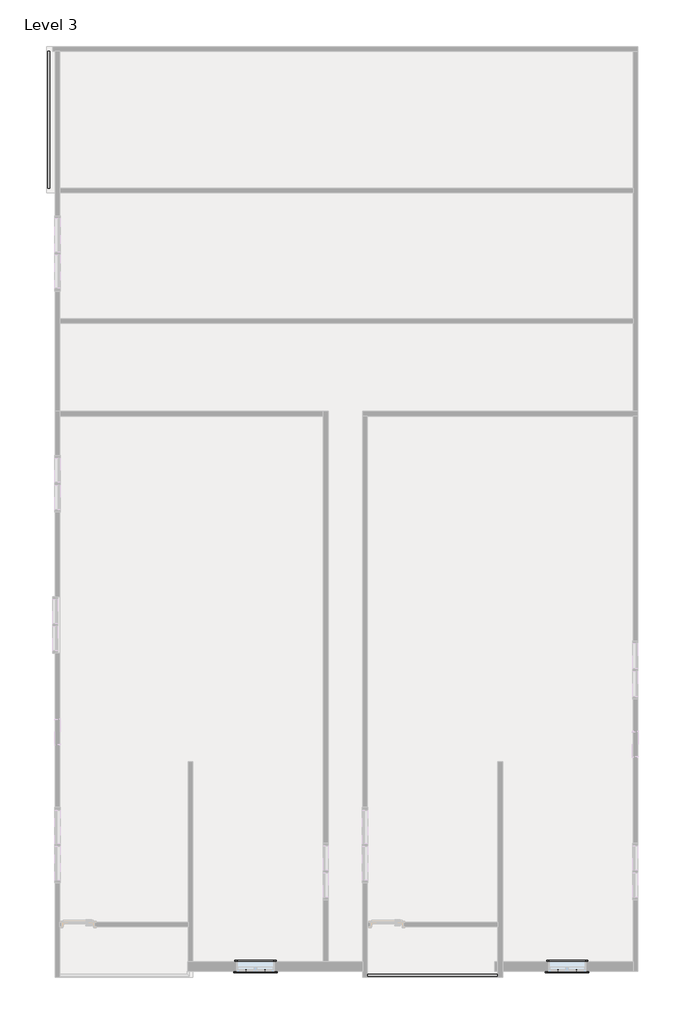
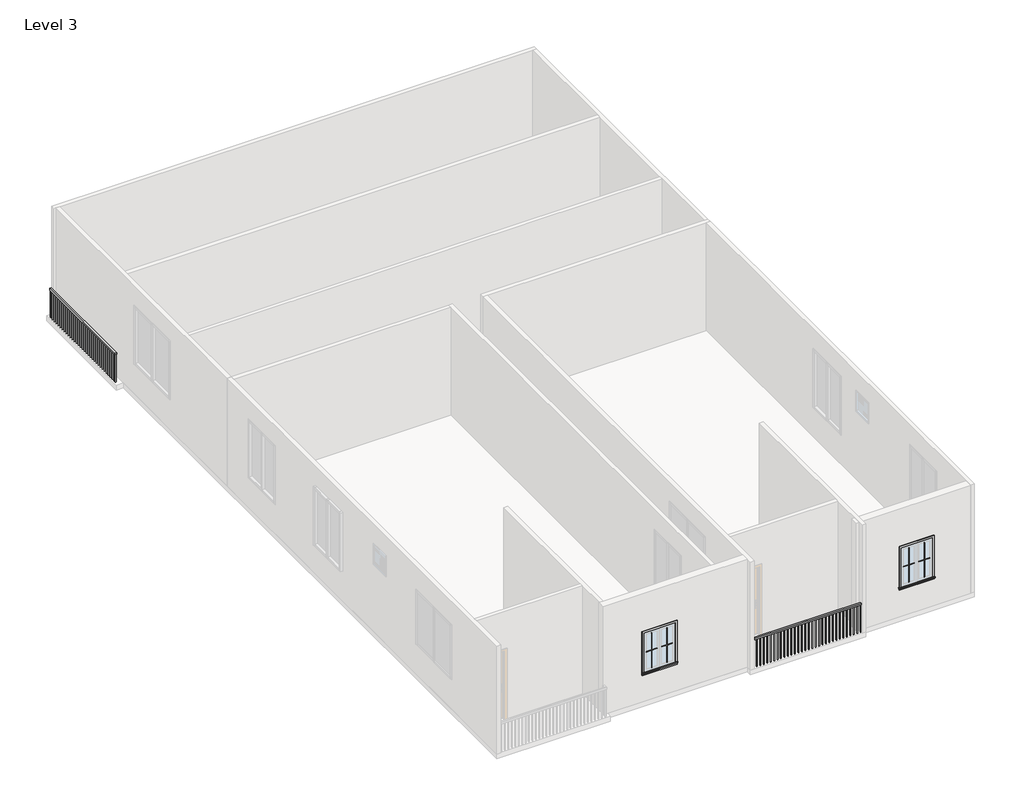
# One storey, part 3 of 3: 8 proxies, 3 railings.
"""IFC4 building model written with IfcOpenShell, lengths in millimetres."""

from ifc_helpers import new_model, si_unit, frame, origin, place, context, project, spatial, polyline, outline, extrude, transform, mapped, element, save
from components import muntin_pattern_2x2_muntin_pattern_2x2_1acec82f, muntin_pattern_2x2_muntin_pattern_2x2_43d02eee, trim_window_exterior_flat_with_sill_e4b28ec3, trim_window_interior_flat_picture_frame_39ff4276

model = new_model("IFC4")

# Units and contexts
model_context = context("Model", 3, world=origin())
ifc_project = project(units=[si_unit("LENGTHUNIT", "METRE", prefix="MILLI")], contexts=[model_context])

# Site, building, storey
site = spatial("IfcSite", under=ifc_project)
building = spatial("IfcBuilding", under=site)
storey = spatial("IfcBuildingStorey", under=building, Name="Level 3", Elevation=6705.6)

# Proxies
placement = place(None, origin())
muntin_pattern_2x2_muntin_pattern_2x2_shape = muntin_pattern_2x2_muntin_pattern_2x2_1acec82f(model_context)
element("IfcBuildingElementProxy", 1, Name="Muntin Pattern_2x2 : Muntin Pattern_2x2", ObjectType="Muntin Pattern_2x2 : Muntin Pattern_2x2", at=placement, inside=storey, context=model_context, shape_type="MappedRepresentation", body=[
    mapped(muntin_pattern_2x2_muntin_pattern_2x2_shape, transform((-3129.6612038, -10576.3529557, 7689.85), x_axis=(-1.0, 0.0, 0.0), y_axis=(0.0, -1.0, 0.0), z_axis=(0.0, 0.0, 1.0))),
])
element("IfcBuildingElementProxy", 2, Name="Muntin Pattern_2x2 : Muntin Pattern_2x2", ObjectType="Muntin Pattern_2x2 : Muntin Pattern_2x2", at=placement, inside=storey, context=model_context, shape_type="MappedRepresentation", body=[
    mapped(muntin_pattern_2x2_muntin_pattern_2x2_shape, transform((4424.1833786, -10576.3529557, 7689.85), x_axis=(-1.0, 0.0, 0.0), y_axis=(0.0, -1.0, 0.0), z_axis=(0.0, 0.0, 1.0))),
])
muntin_pattern_2x2_muntin_pattern_2x2_2_shape = muntin_pattern_2x2_muntin_pattern_2x2_43d02eee(model_context)
element("IfcBuildingElementProxy", 3, Name="Muntin Pattern_2x2 : Muntin Pattern_2x2", ObjectType="Muntin Pattern_2x2 : Muntin Pattern_2x2", at=placement, inside=storey, context=model_context, shape_type="MappedRepresentation", body=[
    mapped(muntin_pattern_2x2_muntin_pattern_2x2_2_shape, transform((-3583.6862038, -10576.3529557, 7689.85), x_axis=(1.0, 0.0, 0.0), y_axis=(0.0, 1.0, 0.0), z_axis=(0.0, 0.0, 1.0))),
])
element("IfcBuildingElementProxy", 4, Name="Muntin Pattern_2x2 : Muntin Pattern_2x2", ObjectType="Muntin Pattern_2x2 : Muntin Pattern_2x2", at=placement, inside=storey, context=model_context, shape_type="MappedRepresentation", body=[
    mapped(muntin_pattern_2x2_muntin_pattern_2x2_2_shape, transform((3970.1583786, -10576.3529557, 7689.85), x_axis=(1.0, 0.0, 0.0), y_axis=(0.0, 1.0, 0.0), z_axis=(0.0, 0.0, 1.0))),
])
trim_window_exterior_flat_with_sill_shape = trim_window_exterior_flat_with_sill_e4b28ec3(model_context)
element("IfcBuildingElementProxy", 5, Name="Trim-Window-Exterior-Flat : with Sill", ObjectType="Trim-Window-Exterior-Flat : with Sill", at=placement, inside=storey, context=model_context, shape_type="MappedRepresentation", body=[
    mapped(trim_window_exterior_flat_with_sill_shape, transform((-3356.6737038, -10585.8779557, 8839.2), x_axis=(1.0, 0.0, 0.0), y_axis=(0.0, 0.0, 1.0), z_axis=(0.0, -1.0, 0.0))),
])
element("IfcBuildingElementProxy", 6, Name="Trim-Window-Exterior-Flat : with Sill", ObjectType="Trim-Window-Exterior-Flat : with Sill", at=placement, inside=storey, context=model_context, shape_type="MappedRepresentation", body=[
    mapped(trim_window_exterior_flat_with_sill_shape, transform((4197.1708786, -10585.8779557, 8839.2), x_axis=(1.0, 0.0, 0.0), y_axis=(0.0, 0.0, 1.0), z_axis=(0.0, -1.0, 0.0))),
])
trim_window_interior_flat_picture_frame_shape = trim_window_interior_flat_picture_frame_39ff4276(model_context)
element("IfcBuildingElementProxy", 7, Name="Trim-Window-Interior-Flat : Picture Frame", ObjectType="Trim-Window-Interior-Flat : Picture Frame", at=placement, inside=storey, context=model_context, shape_type="MappedRepresentation", body=[
    mapped(trim_window_interior_flat_picture_frame_shape, transform((-3356.6737038, -10357.2779557, 8839.2), x_axis=(-1.0, 0.0, 0.0), y_axis=(0.0, 0.0, 1.0), z_axis=(0.0, 1.0, 0.0))),
])
element("IfcBuildingElementProxy", 8, Name="Trim-Window-Interior-Flat : Picture Frame", ObjectType="Trim-Window-Interior-Flat : Picture Frame", at=placement, inside=storey, context=model_context, shape_type="MappedRepresentation", body=[
    mapped(trim_window_interior_flat_picture_frame_shape, transform((4197.1708786, -10357.2779557, 8839.2), x_axis=(-1.0, 0.0, 0.0), y_axis=(0.0, 0.0, 1.0), z_axis=(0.0, 1.0, 0.0))),
])

# Railings
element("IfcRailing", 9, ObjectType="Handrail - Rectangular", at=placement, inside=storey, context=model_context, shape_type="SweptSolid", body=[
    extrude(outline(polyline([(-648.5431282, -10709.8005933), (-648.5431282, -10659.0005933), (2515.990751, -10659.0005933), (2515.990751, -10709.8005933), (-648.5431282, -10709.8005933)])), frame((0.0, 0.0, 7569.2), z_axis=(0.0, 0.0, 1.0), x_axis=(1.0, 0.0, 0.0)), (0.0, 0.0, 1.0), 50.8),
    extrude(outline(polyline([(2491.5318718, -10693.9255933), (2491.5318718, -10674.8755933), (2510.5818718, -10674.8755933), (2510.5818718, -10693.9255933), (2491.5318718, -10693.9255933)])), frame((0.0, 0.0, 6705.6), z_axis=(0.0, 0.0, 1.0), x_axis=(1.0, 0.0, 0.0)), (0.0, 0.0, 1.0), 863.6),
    extrude(outline(polyline([(2389.9318718, -10693.9255933), (2389.9318718, -10674.8755933), (2408.9818718, -10674.8755933), (2408.9818718, -10693.9255933), (2389.9318718, -10693.9255933)])), frame((0.0, 0.0, 6705.6), z_axis=(0.0, 0.0, 1.0), x_axis=(1.0, 0.0, 0.0)), (0.0, 0.0, 1.0), 863.6),
    extrude(outline(polyline([(2288.3318718, -10693.9255933), (2288.3318718, -10674.8755933), (2307.3818718, -10674.8755933), (2307.3818718, -10693.9255933), (2288.3318718, -10693.9255933)])), frame((0.0, 0.0, 6705.6), z_axis=(0.0, 0.0, 1.0), x_axis=(1.0, 0.0, 0.0)), (0.0, 0.0, 1.0), 863.6),
    extrude(outline(polyline([(2186.7318718, -10693.9255933), (2186.7318718, -10674.8755933), (2205.7818718, -10674.8755933), (2205.7818718, -10693.9255933), (2186.7318718, -10693.9255933)])), frame((0.0, 0.0, 6705.6), z_axis=(0.0, 0.0, 1.0), x_axis=(1.0, 0.0, 0.0)), (0.0, 0.0, 1.0), 863.6),
    extrude(outline(polyline([(2085.1318718, -10693.9255933), (2085.1318718, -10674.8755933), (2104.1818718, -10674.8755933), (2104.1818718, -10693.9255933), (2085.1318718, -10693.9255933)])), frame((0.0, 0.0, 6705.6), z_axis=(0.0, 0.0, 1.0), x_axis=(1.0, 0.0, 0.0)), (0.0, 0.0, 1.0), 863.6),
    extrude(outline(polyline([(1983.5318718, -10693.9255933), (1983.5318718, -10674.8755933), (2002.5818718, -10674.8755933), (2002.5818718, -10693.9255933), (1983.5318718, -10693.9255933)])), frame((0.0, 0.0, 6705.6), z_axis=(0.0, 0.0, 1.0), x_axis=(1.0, 0.0, 0.0)), (0.0, 0.0, 1.0), 863.6),
    extrude(outline(polyline([(1881.9318718, -10693.9255933), (1881.9318718, -10674.8755933), (1900.9818718, -10674.8755933), (1900.9818718, -10693.9255933), (1881.9318718, -10693.9255933)])), frame((0.0, 0.0, 6705.6), z_axis=(0.0, 0.0, 1.0), x_axis=(1.0, 0.0, 0.0)), (0.0, 0.0, 1.0), 863.6),
    extrude(outline(polyline([(1780.3318718, -10693.9255933), (1780.3318718, -10674.8755933), (1799.3818718, -10674.8755933), (1799.3818718, -10693.9255933), (1780.3318718, -10693.9255933)])), frame((0.0, 0.0, 6705.6), z_axis=(0.0, 0.0, 1.0), x_axis=(1.0, 0.0, 0.0)), (0.0, 0.0, 1.0), 863.6),
    extrude(outline(polyline([(1678.7318718, -10693.9255933), (1678.7318718, -10674.8755933), (1697.7818718, -10674.8755933), (1697.7818718, -10693.9255933), (1678.7318718, -10693.9255933)])), frame((0.0, 0.0, 6705.6), z_axis=(0.0, 0.0, 1.0), x_axis=(1.0, 0.0, 0.0)), (0.0, 0.0, 1.0), 863.6),
    extrude(outline(polyline([(1577.1318718, -10693.9255933), (1577.1318718, -10674.8755933), (1596.1818718, -10674.8755933), (1596.1818718, -10693.9255933), (1577.1318718, -10693.9255933)])), frame((0.0, 0.0, 6705.6), z_axis=(0.0, 0.0, 1.0), x_axis=(1.0, 0.0, 0.0)), (0.0, 0.0, 1.0), 863.6),
    extrude(outline(polyline([(1475.5318718, -10693.9255933), (1475.5318718, -10674.8755933), (1494.5818718, -10674.8755933), (1494.5818718, -10693.9255933), (1475.5318718, -10693.9255933)])), frame((0.0, 0.0, 6705.6), z_axis=(0.0, 0.0, 1.0), x_axis=(1.0, 0.0, 0.0)), (0.0, 0.0, 1.0), 863.6),
    extrude(outline(polyline([(1373.9318718, -10693.9255933), (1373.9318718, -10674.8755933), (1392.9818718, -10674.8755933), (1392.9818718, -10693.9255933), (1373.9318718, -10693.9255933)])), frame((0.0, 0.0, 6705.6), z_axis=(0.0, 0.0, 1.0), x_axis=(1.0, 0.0, 0.0)), (0.0, 0.0, 1.0), 863.6),
    extrude(outline(polyline([(1272.3318718, -10693.9255933), (1272.3318718, -10674.8755933), (1291.3818718, -10674.8755933), (1291.3818718, -10693.9255933), (1272.3318718, -10693.9255933)])), frame((0.0, 0.0, 6705.6), z_axis=(0.0, 0.0, 1.0), x_axis=(1.0, 0.0, 0.0)), (0.0, 0.0, 1.0), 863.6),
    extrude(outline(polyline([(1170.7318718, -10693.9255933), (1170.7318718, -10674.8755933), (1189.7818718, -10674.8755933), (1189.7818718, -10693.9255933), (1170.7318718, -10693.9255933)])), frame((0.0, 0.0, 6705.6), z_axis=(0.0, 0.0, 1.0), x_axis=(1.0, 0.0, 0.0)), (0.0, 0.0, 1.0), 863.6),
    extrude(outline(polyline([(1069.1318718, -10693.9255933), (1069.1318718, -10674.8755933), (1088.1818718, -10674.8755933), (1088.1818718, -10693.9255933), (1069.1318718, -10693.9255933)])), frame((0.0, 0.0, 6705.6), z_axis=(0.0, 0.0, 1.0), x_axis=(1.0, 0.0, 0.0)), (0.0, 0.0, 1.0), 863.6),
    extrude(outline(polyline([(967.5318718, -10693.9255933), (967.5318718, -10674.8755933), (986.5818718, -10674.8755933), (986.5818718, -10693.9255933), (967.5318718, -10693.9255933)])), frame((0.0, 0.0, 6705.6), z_axis=(0.0, 0.0, 1.0), x_axis=(1.0, 0.0, 0.0)), (0.0, 0.0, 1.0), 863.6),
    extrude(outline(polyline([(865.9318718, -10693.9255933), (865.9318718, -10674.8755933), (884.9818718, -10674.8755933), (884.9818718, -10693.9255933), (865.9318718, -10693.9255933)])), frame((0.0, 0.0, 6705.6), z_axis=(0.0, 0.0, 1.0), x_axis=(1.0, 0.0, 0.0)), (0.0, 0.0, 1.0), 863.6),
    extrude(outline(polyline([(764.3318718, -10693.9255933), (764.3318718, -10674.8755933), (783.3818718, -10674.8755933), (783.3818718, -10693.9255933), (764.3318718, -10693.9255933)])), frame((0.0, 0.0, 6705.6), z_axis=(0.0, 0.0, 1.0), x_axis=(1.0, 0.0, 0.0)), (0.0, 0.0, 1.0), 863.6),
    extrude(outline(polyline([(662.7318718, -10693.9255933), (662.7318718, -10674.8755933), (681.7818718, -10674.8755933), (681.7818718, -10693.9255933), (662.7318718, -10693.9255933)])), frame((0.0, 0.0, 6705.6), z_axis=(0.0, 0.0, 1.0), x_axis=(1.0, 0.0, 0.0)), (0.0, 0.0, 1.0), 863.6),
    extrude(outline(polyline([(561.1318718, -10693.9255933), (561.1318718, -10674.8755933), (580.1818718, -10674.8755933), (580.1818718, -10693.9255933), (561.1318718, -10693.9255933)])), frame((0.0, 0.0, 6705.6), z_axis=(0.0, 0.0, 1.0), x_axis=(1.0, 0.0, 0.0)), (0.0, 0.0, 1.0), 863.6),
    extrude(outline(polyline([(459.5318718, -10693.9255933), (459.5318718, -10674.8755933), (478.5818718, -10674.8755933), (478.5818718, -10693.9255933), (459.5318718, -10693.9255933)])), frame((0.0, 0.0, 6705.6), z_axis=(0.0, 0.0, 1.0), x_axis=(1.0, 0.0, 0.0)), (0.0, 0.0, 1.0), 863.6),
    extrude(outline(polyline([(357.9318718, -10693.9255933), (357.9318718, -10674.8755933), (376.9818718, -10674.8755933), (376.9818718, -10693.9255933), (357.9318718, -10693.9255933)])), frame((0.0, 0.0, 6705.6), z_axis=(0.0, 0.0, 1.0), x_axis=(1.0, 0.0, 0.0)), (0.0, 0.0, 1.0), 863.6),
    extrude(outline(polyline([(256.3318718, -10693.9255933), (256.3318718, -10674.8755933), (275.3818718, -10674.8755933), (275.3818718, -10693.9255933), (256.3318718, -10693.9255933)])), frame((0.0, 0.0, 6705.6), z_axis=(0.0, 0.0, 1.0), x_axis=(1.0, 0.0, 0.0)), (0.0, 0.0, 1.0), 863.6),
    extrude(outline(polyline([(154.7318718, -10693.9255933), (154.7318718, -10674.8755933), (173.7818718, -10674.8755933), (173.7818718, -10693.9255933), (154.7318718, -10693.9255933)])), frame((0.0, 0.0, 6705.6), z_axis=(0.0, 0.0, 1.0), x_axis=(1.0, 0.0, 0.0)), (0.0, 0.0, 1.0), 863.6),
    extrude(outline(polyline([(53.1318718, -10693.9255933), (53.1318718, -10674.8755933), (72.1818718, -10674.8755933), (72.1818718, -10693.9255933), (53.1318718, -10693.9255933)])), frame((0.0, 0.0, 6705.6), z_axis=(0.0, 0.0, 1.0), x_axis=(1.0, 0.0, 0.0)), (0.0, 0.0, 1.0), 863.6),
    extrude(outline(polyline([(-48.4681282, -10693.9255933), (-48.4681282, -10674.8755933), (-29.4181282, -10674.8755933), (-29.4181282, -10693.9255933), (-48.4681282, -10693.9255933)])), frame((0.0, 0.0, 6705.6), z_axis=(0.0, 0.0, 1.0), x_axis=(1.0, 0.0, 0.0)), (0.0, 0.0, 1.0), 863.6),
    extrude(outline(polyline([(-150.0681282, -10693.9255933), (-150.0681282, -10674.8755933), (-131.0181282, -10674.8755933), (-131.0181282, -10693.9255933), (-150.0681282, -10693.9255933)])), frame((0.0, 0.0, 6705.6), z_axis=(0.0, 0.0, 1.0), x_axis=(1.0, 0.0, 0.0)), (0.0, 0.0, 1.0), 863.6),
    extrude(outline(polyline([(-251.6681282, -10693.9255933), (-251.6681282, -10674.8755933), (-232.6181282, -10674.8755933), (-232.6181282, -10693.9255933), (-251.6681282, -10693.9255933)])), frame((0.0, 0.0, 6705.6), z_axis=(0.0, 0.0, 1.0), x_axis=(1.0, 0.0, 0.0)), (0.0, 0.0, 1.0), 863.6),
    extrude(outline(polyline([(-353.2681282, -10693.9255933), (-353.2681282, -10674.8755933), (-334.2181282, -10674.8755933), (-334.2181282, -10693.9255933), (-353.2681282, -10693.9255933)])), frame((0.0, 0.0, 6705.6), z_axis=(0.0, 0.0, 1.0), x_axis=(1.0, 0.0, 0.0)), (0.0, 0.0, 1.0), 863.6),
    extrude(outline(polyline([(-454.8681282, -10693.9255933), (-454.8681282, -10674.8755933), (-435.8181282, -10674.8755933), (-435.8181282, -10693.9255933), (-454.8681282, -10693.9255933)])), frame((0.0, 0.0, 6705.6), z_axis=(0.0, 0.0, 1.0), x_axis=(1.0, 0.0, 0.0)), (0.0, 0.0, 1.0), 863.6),
    extrude(outline(polyline([(-556.4681282, -10693.9255933), (-556.4681282, -10674.8755933), (-537.4181282, -10674.8755933), (-537.4181282, -10693.9255933), (-556.4681282, -10693.9255933)])), frame((0.0, 0.0, 6705.6), z_axis=(0.0, 0.0, 1.0), x_axis=(1.0, 0.0, 0.0)), (0.0, 0.0, 1.0), 863.6),
    extrude(outline(polyline([(2496.940751, -10693.9255933), (2496.940751, -10674.8755933), (2515.990751, -10674.8755933), (2515.990751, -10693.9255933), (2496.940751, -10693.9255933)])), frame((0.0, 0.0, 6705.6), z_axis=(0.0, 0.0, 1.0), x_axis=(1.0, 0.0, 0.0)), (0.0, 0.0, 1.0), 863.6),
    extrude(outline(polyline([(-648.5431282, -10693.9255933), (-648.5431282, -10674.8755933), (-629.4931282, -10674.8755933), (-629.4931282, -10693.9255933), (-648.5431282, -10693.9255933)])), frame((0.0, 0.0, 6705.6), z_axis=(0.0, 0.0, 1.0), x_axis=(1.0, 0.0, 0.0)), (0.0, 0.0, 1.0), 863.6),
])
element("IfcRailing", 10, ObjectType="Handrail - Rectangular", at=placement, inside=storey, context=model_context, shape_type="SweptSolid", body=[
    extrude(outline(polyline([(-8391.7551246, 11703.9189683), (-8340.9551246, 11703.9189683), (-8340.9551246, 8387.4224771), (-8391.7551246, 8387.4224771), (-8391.7551246, 11703.9189683)])), frame((0.0, 0.0, 7569.2), z_axis=(0.0, 0.0, 1.0), x_axis=(1.0, 0.0, 0.0)), (0.0, 0.0, 1.0), 50.8),
    extrude(outline(polyline([(-8375.8801246, 8462.2439683), (-8356.8301246, 8462.2439683), (-8356.8301246, 8443.1939683), (-8375.8801246, 8443.1939683), (-8375.8801246, 8462.2439683)])), frame((0.0, 0.0, 6705.6), z_axis=(0.0, 0.0, 1.0), x_axis=(1.0, 0.0, 0.0)), (0.0, 0.0, 1.0), 863.6),
    extrude(outline(polyline([(-8375.8801246, 8563.8439683), (-8356.8301246, 8563.8439683), (-8356.8301246, 8544.7939683), (-8375.8801246, 8544.7939683), (-8375.8801246, 8563.8439683)])), frame((0.0, 0.0, 6705.6), z_axis=(0.0, 0.0, 1.0), x_axis=(1.0, 0.0, 0.0)), (0.0, 0.0, 1.0), 863.6),
    extrude(outline(polyline([(-8375.8801246, 8665.4439683), (-8356.8301246, 8665.4439683), (-8356.8301246, 8646.3939683), (-8375.8801246, 8646.3939683), (-8375.8801246, 8665.4439683)])), frame((0.0, 0.0, 6705.6), z_axis=(0.0, 0.0, 1.0), x_axis=(1.0, 0.0, 0.0)), (0.0, 0.0, 1.0), 863.6),
    extrude(outline(polyline([(-8375.8801246, 8767.0439683), (-8356.8301246, 8767.0439683), (-8356.8301246, 8747.9939683), (-8375.8801246, 8747.9939683), (-8375.8801246, 8767.0439683)])), frame((0.0, 0.0, 6705.6), z_axis=(0.0, 0.0, 1.0), x_axis=(1.0, 0.0, 0.0)), (0.0, 0.0, 1.0), 863.6),
    extrude(outline(polyline([(-8375.8801246, 8868.6439683), (-8356.8301246, 8868.6439683), (-8356.8301246, 8849.5939683), (-8375.8801246, 8849.5939683), (-8375.8801246, 8868.6439683)])), frame((0.0, 0.0, 6705.6), z_axis=(0.0, 0.0, 1.0), x_axis=(1.0, 0.0, 0.0)), (0.0, 0.0, 1.0), 863.6),
    extrude(outline(polyline([(-8375.8801246, 8970.2439683), (-8356.8301246, 8970.2439683), (-8356.8301246, 8951.1939683), (-8375.8801246, 8951.1939683), (-8375.8801246, 8970.2439683)])), frame((0.0, 0.0, 6705.6), z_axis=(0.0, 0.0, 1.0), x_axis=(1.0, 0.0, 0.0)), (0.0, 0.0, 1.0), 863.6),
    extrude(outline(polyline([(-8375.8801246, 9071.8439683), (-8356.8301246, 9071.8439683), (-8356.8301246, 9052.7939683), (-8375.8801246, 9052.7939683), (-8375.8801246, 9071.8439683)])), frame((0.0, 0.0, 6705.6), z_axis=(0.0, 0.0, 1.0), x_axis=(1.0, 0.0, 0.0)), (0.0, 0.0, 1.0), 863.6),
    extrude(outline(polyline([(-8375.8801246, 9173.4439683), (-8356.8301246, 9173.4439683), (-8356.8301246, 9154.3939683), (-8375.8801246, 9154.3939683), (-8375.8801246, 9173.4439683)])), frame((0.0, 0.0, 6705.6), z_axis=(0.0, 0.0, 1.0), x_axis=(1.0, 0.0, 0.0)), (0.0, 0.0, 1.0), 863.6),
    extrude(outline(polyline([(-8375.8801246, 9275.0439683), (-8356.8301246, 9275.0439683), (-8356.8301246, 9255.9939683), (-8375.8801246, 9255.9939683), (-8375.8801246, 9275.0439683)])), frame((0.0, 0.0, 6705.6), z_axis=(0.0, 0.0, 1.0), x_axis=(1.0, 0.0, 0.0)), (0.0, 0.0, 1.0), 863.6),
    extrude(outline(polyline([(-8375.8801246, 9376.6439683), (-8356.8301246, 9376.6439683), (-8356.8301246, 9357.5939683), (-8375.8801246, 9357.5939683), (-8375.8801246, 9376.6439683)])), frame((0.0, 0.0, 6705.6), z_axis=(0.0, 0.0, 1.0), x_axis=(1.0, 0.0, 0.0)), (0.0, 0.0, 1.0), 863.6),
    extrude(outline(polyline([(-8375.8801246, 9478.2439683), (-8356.8301246, 9478.2439683), (-8356.8301246, 9459.1939683), (-8375.8801246, 9459.1939683), (-8375.8801246, 9478.2439683)])), frame((0.0, 0.0, 6705.6), z_axis=(0.0, 0.0, 1.0), x_axis=(1.0, 0.0, 0.0)), (0.0, 0.0, 1.0), 863.6),
    extrude(outline(polyline([(-8375.8801246, 9579.8439683), (-8356.8301246, 9579.8439683), (-8356.8301246, 9560.7939683), (-8375.8801246, 9560.7939683), (-8375.8801246, 9579.8439683)])), frame((0.0, 0.0, 6705.6), z_axis=(0.0, 0.0, 1.0), x_axis=(1.0, 0.0, 0.0)), (0.0, 0.0, 1.0), 863.6),
    extrude(outline(polyline([(-8375.8801246, 9681.4439683), (-8356.8301246, 9681.4439683), (-8356.8301246, 9662.3939683), (-8375.8801246, 9662.3939683), (-8375.8801246, 9681.4439683)])), frame((0.0, 0.0, 6705.6), z_axis=(0.0, 0.0, 1.0), x_axis=(1.0, 0.0, 0.0)), (0.0, 0.0, 1.0), 863.6),
    extrude(outline(polyline([(-8375.8801246, 9783.0439683), (-8356.8301246, 9783.0439683), (-8356.8301246, 9763.9939683), (-8375.8801246, 9763.9939683), (-8375.8801246, 9783.0439683)])), frame((0.0, 0.0, 6705.6), z_axis=(0.0, 0.0, 1.0), x_axis=(1.0, 0.0, 0.0)), (0.0, 0.0, 1.0), 863.6),
    extrude(outline(polyline([(-8375.8801246, 9884.6439683), (-8356.8301246, 9884.6439683), (-8356.8301246, 9865.5939683), (-8375.8801246, 9865.5939683), (-8375.8801246, 9884.6439683)])), frame((0.0, 0.0, 6705.6), z_axis=(0.0, 0.0, 1.0), x_axis=(1.0, 0.0, 0.0)), (0.0, 0.0, 1.0), 863.6),
    extrude(outline(polyline([(-8375.8801246, 9986.2439683), (-8356.8301246, 9986.2439683), (-8356.8301246, 9967.1939683), (-8375.8801246, 9967.1939683), (-8375.8801246, 9986.2439683)])), frame((0.0, 0.0, 6705.6), z_axis=(0.0, 0.0, 1.0), x_axis=(1.0, 0.0, 0.0)), (0.0, 0.0, 1.0), 863.6),
    extrude(outline(polyline([(-8375.8801246, 10087.8439683), (-8356.8301246, 10087.8439683), (-8356.8301246, 10068.7939683), (-8375.8801246, 10068.7939683), (-8375.8801246, 10087.8439683)])), frame((0.0, 0.0, 6705.6), z_axis=(0.0, 0.0, 1.0), x_axis=(1.0, 0.0, 0.0)), (0.0, 0.0, 1.0), 863.6),
    extrude(outline(polyline([(-8375.8801246, 10189.4439683), (-8356.8301246, 10189.4439683), (-8356.8301246, 10170.3939683), (-8375.8801246, 10170.3939683), (-8375.8801246, 10189.4439683)])), frame((0.0, 0.0, 6705.6), z_axis=(0.0, 0.0, 1.0), x_axis=(1.0, 0.0, 0.0)), (0.0, 0.0, 1.0), 863.6),
    extrude(outline(polyline([(-8375.8801246, 10291.0439683), (-8356.8301246, 10291.0439683), (-8356.8301246, 10271.9939683), (-8375.8801246, 10271.9939683), (-8375.8801246, 10291.0439683)])), frame((0.0, 0.0, 6705.6), z_axis=(0.0, 0.0, 1.0), x_axis=(1.0, 0.0, 0.0)), (0.0, 0.0, 1.0), 863.6),
    extrude(outline(polyline([(-8375.8801246, 10392.6439683), (-8356.8301246, 10392.6439683), (-8356.8301246, 10373.5939683), (-8375.8801246, 10373.5939683), (-8375.8801246, 10392.6439683)])), frame((0.0, 0.0, 6705.6), z_axis=(0.0, 0.0, 1.0), x_axis=(1.0, 0.0, 0.0)), (0.0, 0.0, 1.0), 863.6),
    extrude(outline(polyline([(-8375.8801246, 10494.2439683), (-8356.8301246, 10494.2439683), (-8356.8301246, 10475.1939683), (-8375.8801246, 10475.1939683), (-8375.8801246, 10494.2439683)])), frame((0.0, 0.0, 6705.6), z_axis=(0.0, 0.0, 1.0), x_axis=(1.0, 0.0, 0.0)), (0.0, 0.0, 1.0), 863.6),
    extrude(outline(polyline([(-8375.8801246, 10595.8439683), (-8356.8301246, 10595.8439683), (-8356.8301246, 10576.7939683), (-8375.8801246, 10576.7939683), (-8375.8801246, 10595.8439683)])), frame((0.0, 0.0, 6705.6), z_axis=(0.0, 0.0, 1.0), x_axis=(1.0, 0.0, 0.0)), (0.0, 0.0, 1.0), 863.6),
    extrude(outline(polyline([(-8375.8801246, 10697.4439683), (-8356.8301246, 10697.4439683), (-8356.8301246, 10678.3939683), (-8375.8801246, 10678.3939683), (-8375.8801246, 10697.4439683)])), frame((0.0, 0.0, 6705.6), z_axis=(0.0, 0.0, 1.0), x_axis=(1.0, 0.0, 0.0)), (0.0, 0.0, 1.0), 863.6),
    extrude(outline(polyline([(-8375.8801246, 10799.0439683), (-8356.8301246, 10799.0439683), (-8356.8301246, 10779.9939683), (-8375.8801246, 10779.9939683), (-8375.8801246, 10799.0439683)])), frame((0.0, 0.0, 6705.6), z_axis=(0.0, 0.0, 1.0), x_axis=(1.0, 0.0, 0.0)), (0.0, 0.0, 1.0), 863.6),
    extrude(outline(polyline([(-8375.8801246, 10900.6439683), (-8356.8301246, 10900.6439683), (-8356.8301246, 10881.5939683), (-8375.8801246, 10881.5939683), (-8375.8801246, 10900.6439683)])), frame((0.0, 0.0, 6705.6), z_axis=(0.0, 0.0, 1.0), x_axis=(1.0, 0.0, 0.0)), (0.0, 0.0, 1.0), 863.6),
    extrude(outline(polyline([(-8375.8801246, 11002.2439683), (-8356.8301246, 11002.2439683), (-8356.8301246, 10983.1939683), (-8375.8801246, 10983.1939683), (-8375.8801246, 11002.2439683)])), frame((0.0, 0.0, 6705.6), z_axis=(0.0, 0.0, 1.0), x_axis=(1.0, 0.0, 0.0)), (0.0, 0.0, 1.0), 863.6),
    extrude(outline(polyline([(-8375.8801246, 11103.8439683), (-8356.8301246, 11103.8439683), (-8356.8301246, 11084.7939683), (-8375.8801246, 11084.7939683), (-8375.8801246, 11103.8439683)])), frame((0.0, 0.0, 6705.6), z_axis=(0.0, 0.0, 1.0), x_axis=(1.0, 0.0, 0.0)), (0.0, 0.0, 1.0), 863.6),
    extrude(outline(polyline([(-8375.8801246, 11205.4439683), (-8356.8301246, 11205.4439683), (-8356.8301246, 11186.3939683), (-8375.8801246, 11186.3939683), (-8375.8801246, 11205.4439683)])), frame((0.0, 0.0, 6705.6), z_axis=(0.0, 0.0, 1.0), x_axis=(1.0, 0.0, 0.0)), (0.0, 0.0, 1.0), 863.6),
    extrude(outline(polyline([(-8375.8801246, 11307.0439683), (-8356.8301246, 11307.0439683), (-8356.8301246, 11287.9939683), (-8375.8801246, 11287.9939683), (-8375.8801246, 11307.0439683)])), frame((0.0, 0.0, 6705.6), z_axis=(0.0, 0.0, 1.0), x_axis=(1.0, 0.0, 0.0)), (0.0, 0.0, 1.0), 863.6),
    extrude(outline(polyline([(-8375.8801246, 11408.6439683), (-8356.8301246, 11408.6439683), (-8356.8301246, 11389.5939683), (-8375.8801246, 11389.5939683), (-8375.8801246, 11408.6439683)])), frame((0.0, 0.0, 6705.6), z_axis=(0.0, 0.0, 1.0), x_axis=(1.0, 0.0, 0.0)), (0.0, 0.0, 1.0), 863.6),
    extrude(outline(polyline([(-8375.8801246, 11510.2439683), (-8356.8301246, 11510.2439683), (-8356.8301246, 11491.1939683), (-8375.8801246, 11491.1939683), (-8375.8801246, 11510.2439683)])), frame((0.0, 0.0, 6705.6), z_axis=(0.0, 0.0, 1.0), x_axis=(1.0, 0.0, 0.0)), (0.0, 0.0, 1.0), 863.6),
    extrude(outline(polyline([(-8375.8801246, 11611.8439683), (-8356.8301246, 11611.8439683), (-8356.8301246, 11592.7939683), (-8375.8801246, 11592.7939683), (-8375.8801246, 11611.8439683)])), frame((0.0, 0.0, 6705.6), z_axis=(0.0, 0.0, 1.0), x_axis=(1.0, 0.0, 0.0)), (0.0, 0.0, 1.0), 863.6),
    extrude(outline(polyline([(-8375.8801246, 8406.4724771), (-8356.8301246, 8406.4724771), (-8356.8301246, 8387.4224771), (-8375.8801246, 8387.4224771), (-8375.8801246, 8406.4724771)])), frame((0.0, 0.0, 6705.6), z_axis=(0.0, 0.0, 1.0), x_axis=(1.0, 0.0, 0.0)), (0.0, 0.0, 1.0), 863.6),
    extrude(outline(polyline([(-8375.8801246, 11703.9189683), (-8356.8301246, 11703.9189683), (-8356.8301246, 11684.8689683), (-8375.8801246, 11684.8689683), (-8375.8801246, 11703.9189683)])), frame((0.0, 0.0, 6705.6), z_axis=(0.0, 0.0, 1.0), x_axis=(1.0, 0.0, 0.0)), (0.0, 0.0, 1.0), 863.6),
])
element("IfcRailing", 11, ObjectType="Handrail - Rectangular", at=placement, inside=storey, context=model_context, shape_type="SweptSolid", body=[
    extrude(outline(polyline([(5830.4721078, 11594.1725279), (5881.2721078, 11594.1725279), (5881.2721078, 8505.5262287), (5830.4721078, 8505.5262287), (5830.4721078, 11594.1725279)])), frame((0.0, 0.0, 7569.2), z_axis=(0.0, 0.0, 1.0), x_axis=(1.0, 0.0, 0.0)), (0.0, 0.0, 1.0), 50.8),
    extrude(outline(polyline([(5846.3471078, 8555.6975279), (5865.3971078, 8555.6975279), (5865.3971078, 8536.6475279), (5846.3471078, 8536.6475279), (5846.3471078, 8555.6975279)])), frame((0.0, 0.0, 6705.6), z_axis=(0.0, 0.0, 1.0), x_axis=(1.0, 0.0, 0.0)), (0.0, 0.0, 1.0), 863.6),
    extrude(outline(polyline([(5846.3471078, 8657.2975279), (5865.3971078, 8657.2975279), (5865.3971078, 8638.2475279), (5846.3471078, 8638.2475279), (5846.3471078, 8657.2975279)])), frame((0.0, 0.0, 6705.6), z_axis=(0.0, 0.0, 1.0), x_axis=(1.0, 0.0, 0.0)), (0.0, 0.0, 1.0), 863.6),
    extrude(outline(polyline([(5846.3471078, 8758.8975279), (5865.3971078, 8758.8975279), (5865.3971078, 8739.8475279), (5846.3471078, 8739.8475279), (5846.3471078, 8758.8975279)])), frame((0.0, 0.0, 6705.6), z_axis=(0.0, 0.0, 1.0), x_axis=(1.0, 0.0, 0.0)), (0.0, 0.0, 1.0), 863.6),
    extrude(outline(polyline([(5846.3471078, 8860.4975279), (5865.3971078, 8860.4975279), (5865.3971078, 8841.4475279), (5846.3471078, 8841.4475279), (5846.3471078, 8860.4975279)])), frame((0.0, 0.0, 6705.6), z_axis=(0.0, 0.0, 1.0), x_axis=(1.0, 0.0, 0.0)), (0.0, 0.0, 1.0), 863.6),
    extrude(outline(polyline([(5846.3471078, 8962.0975279), (5865.3971078, 8962.0975279), (5865.3971078, 8943.0475279), (5846.3471078, 8943.0475279), (5846.3471078, 8962.0975279)])), frame((0.0, 0.0, 6705.6), z_axis=(0.0, 0.0, 1.0), x_axis=(1.0, 0.0, 0.0)), (0.0, 0.0, 1.0), 863.6),
    extrude(outline(polyline([(5846.3471078, 9063.6975279), (5865.3971078, 9063.6975279), (5865.3971078, 9044.6475279), (5846.3471078, 9044.6475279), (5846.3471078, 9063.6975279)])), frame((0.0, 0.0, 6705.6), z_axis=(0.0, 0.0, 1.0), x_axis=(1.0, 0.0, 0.0)), (0.0, 0.0, 1.0), 863.6),
    extrude(outline(polyline([(5846.3471078, 9165.2975279), (5865.3971078, 9165.2975279), (5865.3971078, 9146.2475279), (5846.3471078, 9146.2475279), (5846.3471078, 9165.2975279)])), frame((0.0, 0.0, 6705.6), z_axis=(0.0, 0.0, 1.0), x_axis=(1.0, 0.0, 0.0)), (0.0, 0.0, 1.0), 863.6),
    extrude(outline(polyline([(5846.3471078, 9266.8975279), (5865.3971078, 9266.8975279), (5865.3971078, 9247.8475279), (5846.3471078, 9247.8475279), (5846.3471078, 9266.8975279)])), frame((0.0, 0.0, 6705.6), z_axis=(0.0, 0.0, 1.0), x_axis=(1.0, 0.0, 0.0)), (0.0, 0.0, 1.0), 863.6),
    extrude(outline(polyline([(5846.3471078, 9368.4975279), (5865.3971078, 9368.4975279), (5865.3971078, 9349.4475279), (5846.3471078, 9349.4475279), (5846.3471078, 9368.4975279)])), frame((0.0, 0.0, 6705.6), z_axis=(0.0, 0.0, 1.0), x_axis=(1.0, 0.0, 0.0)), (0.0, 0.0, 1.0), 863.6),
    extrude(outline(polyline([(5846.3471078, 9470.0975279), (5865.3971078, 9470.0975279), (5865.3971078, 9451.0475279), (5846.3471078, 9451.0475279), (5846.3471078, 9470.0975279)])), frame((0.0, 0.0, 6705.6), z_axis=(0.0, 0.0, 1.0), x_axis=(1.0, 0.0, 0.0)), (0.0, 0.0, 1.0), 863.6),
    extrude(outline(polyline([(5846.3471078, 9571.6975279), (5865.3971078, 9571.6975279), (5865.3971078, 9552.6475279), (5846.3471078, 9552.6475279), (5846.3471078, 9571.6975279)])), frame((0.0, 0.0, 6705.6), z_axis=(0.0, 0.0, 1.0), x_axis=(1.0, 0.0, 0.0)), (0.0, 0.0, 1.0), 863.6),
    extrude(outline(polyline([(5846.3471078, 9673.2975279), (5865.3971078, 9673.2975279), (5865.3971078, 9654.2475279), (5846.3471078, 9654.2475279), (5846.3471078, 9673.2975279)])), frame((0.0, 0.0, 6705.6), z_axis=(0.0, 0.0, 1.0), x_axis=(1.0, 0.0, 0.0)), (0.0, 0.0, 1.0), 863.6),
    extrude(outline(polyline([(5846.3471078, 9774.8975279), (5865.3971078, 9774.8975279), (5865.3971078, 9755.8475279), (5846.3471078, 9755.8475279), (5846.3471078, 9774.8975279)])), frame((0.0, 0.0, 6705.6), z_axis=(0.0, 0.0, 1.0), x_axis=(1.0, 0.0, 0.0)), (0.0, 0.0, 1.0), 863.6),
    extrude(outline(polyline([(5846.3471078, 9876.4975279), (5865.3971078, 9876.4975279), (5865.3971078, 9857.4475279), (5846.3471078, 9857.4475279), (5846.3471078, 9876.4975279)])), frame((0.0, 0.0, 6705.6), z_axis=(0.0, 0.0, 1.0), x_axis=(1.0, 0.0, 0.0)), (0.0, 0.0, 1.0), 863.6),
    extrude(outline(polyline([(5846.3471078, 9978.0975279), (5865.3971078, 9978.0975279), (5865.3971078, 9959.0475279), (5846.3471078, 9959.0475279), (5846.3471078, 9978.0975279)])), frame((0.0, 0.0, 6705.6), z_axis=(0.0, 0.0, 1.0), x_axis=(1.0, 0.0, 0.0)), (0.0, 0.0, 1.0), 863.6),
    extrude(outline(polyline([(5846.3471078, 10079.6975279), (5865.3971078, 10079.6975279), (5865.3971078, 10060.6475279), (5846.3471078, 10060.6475279), (5846.3471078, 10079.6975279)])), frame((0.0, 0.0, 6705.6), z_axis=(0.0, 0.0, 1.0), x_axis=(1.0, 0.0, 0.0)), (0.0, 0.0, 1.0), 863.6),
    extrude(outline(polyline([(5846.3471078, 10181.2975279), (5865.3971078, 10181.2975279), (5865.3971078, 10162.2475279), (5846.3471078, 10162.2475279), (5846.3471078, 10181.2975279)])), frame((0.0, 0.0, 6705.6), z_axis=(0.0, 0.0, 1.0), x_axis=(1.0, 0.0, 0.0)), (0.0, 0.0, 1.0), 863.6),
    extrude(outline(polyline([(5846.3471078, 10282.8975279), (5865.3971078, 10282.8975279), (5865.3971078, 10263.8475279), (5846.3471078, 10263.8475279), (5846.3471078, 10282.8975279)])), frame((0.0, 0.0, 6705.6), z_axis=(0.0, 0.0, 1.0), x_axis=(1.0, 0.0, 0.0)), (0.0, 0.0, 1.0), 863.6),
    extrude(outline(polyline([(5846.3471078, 10384.4975279), (5865.3971078, 10384.4975279), (5865.3971078, 10365.4475279), (5846.3471078, 10365.4475279), (5846.3471078, 10384.4975279)])), frame((0.0, 0.0, 6705.6), z_axis=(0.0, 0.0, 1.0), x_axis=(1.0, 0.0, 0.0)), (0.0, 0.0, 1.0), 863.6),
    extrude(outline(polyline([(5846.3471078, 10486.0975279), (5865.3971078, 10486.0975279), (5865.3971078, 10467.0475279), (5846.3471078, 10467.0475279), (5846.3471078, 10486.0975279)])), frame((0.0, 0.0, 6705.6), z_axis=(0.0, 0.0, 1.0), x_axis=(1.0, 0.0, 0.0)), (0.0, 0.0, 1.0), 863.6),
    extrude(outline(polyline([(5846.3471078, 10587.6975279), (5865.3971078, 10587.6975279), (5865.3971078, 10568.6475279), (5846.3471078, 10568.6475279), (5846.3471078, 10587.6975279)])), frame((0.0, 0.0, 6705.6), z_axis=(0.0, 0.0, 1.0), x_axis=(1.0, 0.0, 0.0)), (0.0, 0.0, 1.0), 863.6),
    extrude(outline(polyline([(5846.3471078, 10689.2975279), (5865.3971078, 10689.2975279), (5865.3971078, 10670.2475279), (5846.3471078, 10670.2475279), (5846.3471078, 10689.2975279)])), frame((0.0, 0.0, 6705.6), z_axis=(0.0, 0.0, 1.0), x_axis=(1.0, 0.0, 0.0)), (0.0, 0.0, 1.0), 863.6),
    extrude(outline(polyline([(5846.3471078, 10790.8975279), (5865.3971078, 10790.8975279), (5865.3971078, 10771.8475279), (5846.3471078, 10771.8475279), (5846.3471078, 10790.8975279)])), frame((0.0, 0.0, 6705.6), z_axis=(0.0, 0.0, 1.0), x_axis=(1.0, 0.0, 0.0)), (0.0, 0.0, 1.0), 863.6),
    extrude(outline(polyline([(5846.3471078, 10892.4975279), (5865.3971078, 10892.4975279), (5865.3971078, 10873.4475279), (5846.3471078, 10873.4475279), (5846.3471078, 10892.4975279)])), frame((0.0, 0.0, 6705.6), z_axis=(0.0, 0.0, 1.0), x_axis=(1.0, 0.0, 0.0)), (0.0, 0.0, 1.0), 863.6),
    extrude(outline(polyline([(5846.3471078, 10994.0975279), (5865.3971078, 10994.0975279), (5865.3971078, 10975.0475279), (5846.3471078, 10975.0475279), (5846.3471078, 10994.0975279)])), frame((0.0, 0.0, 6705.6), z_axis=(0.0, 0.0, 1.0), x_axis=(1.0, 0.0, 0.0)), (0.0, 0.0, 1.0), 863.6),
    extrude(outline(polyline([(5846.3471078, 11095.6975279), (5865.3971078, 11095.6975279), (5865.3971078, 11076.6475279), (5846.3471078, 11076.6475279), (5846.3471078, 11095.6975279)])), frame((0.0, 0.0, 6705.6), z_axis=(0.0, 0.0, 1.0), x_axis=(1.0, 0.0, 0.0)), (0.0, 0.0, 1.0), 863.6),
    extrude(outline(polyline([(5846.3471078, 11197.2975279), (5865.3971078, 11197.2975279), (5865.3971078, 11178.2475279), (5846.3471078, 11178.2475279), (5846.3471078, 11197.2975279)])), frame((0.0, 0.0, 6705.6), z_axis=(0.0, 0.0, 1.0), x_axis=(1.0, 0.0, 0.0)), (0.0, 0.0, 1.0), 863.6),
    extrude(outline(polyline([(5846.3471078, 11298.8975279), (5865.3971078, 11298.8975279), (5865.3971078, 11279.8475279), (5846.3471078, 11279.8475279), (5846.3471078, 11298.8975279)])), frame((0.0, 0.0, 6705.6), z_axis=(0.0, 0.0, 1.0), x_axis=(1.0, 0.0, 0.0)), (0.0, 0.0, 1.0), 863.6),
    extrude(outline(polyline([(5846.3471078, 11400.4975279), (5865.3971078, 11400.4975279), (5865.3971078, 11381.4475279), (5846.3471078, 11381.4475279), (5846.3471078, 11400.4975279)])), frame((0.0, 0.0, 6705.6), z_axis=(0.0, 0.0, 1.0), x_axis=(1.0, 0.0, 0.0)), (0.0, 0.0, 1.0), 863.6),
    extrude(outline(polyline([(5846.3471078, 11502.0975279), (5865.3971078, 11502.0975279), (5865.3971078, 11483.0475279), (5846.3471078, 11483.0475279), (5846.3471078, 11502.0975279)])), frame((0.0, 0.0, 6705.6), z_axis=(0.0, 0.0, 1.0), x_axis=(1.0, 0.0, 0.0)), (0.0, 0.0, 1.0), 863.6),
    extrude(outline(polyline([(5846.3471078, 8524.5762287), (5865.3971078, 8524.5762287), (5865.3971078, 8505.5262287), (5846.3471078, 8505.5262287), (5846.3471078, 8524.5762287)])), frame((0.0, 0.0, 6705.6), z_axis=(0.0, 0.0, 1.0), x_axis=(1.0, 0.0, 0.0)), (0.0, 0.0, 1.0), 863.6),
    extrude(outline(polyline([(5846.3471078, 11594.1725279), (5865.3971078, 11594.1725279), (5865.3971078, 11575.1225279), (5846.3471078, 11575.1225279), (5846.3471078, 11594.1725279)])), frame((0.0, 0.0, 6705.6), z_axis=(0.0, 0.0, 1.0), x_axis=(1.0, 0.0, 0.0)), (0.0, 0.0, 1.0), 863.6),
])

save(model, "model.ifc")

# Revit data of these elements
# Type "Muntin Pattern_2x2 : Muntin Pattern_2x2"
#   Width [instance default] = 4' - 0"
#   Thickness = 0' - 0 1/2"
#   Height [instance default] = 4' - 0"
#   Distance = 0' - 0 3/4"
#   Interior Material [instance default] = none
#   Exterior Material [instance default] = none
#   Default Elevation = 0
# Type "Trim-Window-Exterior-Flat : with Sill"
#   Trim Width = 0' - 2 1/4"
#   Trim Thickness_Picture Frame = 0' - 1 1/4"
#   Trim Thickness_with Sill = 0' - 0 3/4"
#   Sill Thickness = 0' - 1 1/4"
#   Opening Width [instance default] = 2' - 0"
#   Opening Height [instance default] = 3' - 0"
#   Default Elevation = 4' - 0"
#   Sill = yes
#   Picture Frame = no
#   Trim Material [instance default] = none
# Type "Trim-Window-Interior-Flat : Picture Frame"
#   Trim Thickness_Picture Frame = 0' - 1 1/4"
#   Trim Width = 0' - 2 1/4"
#   Trim Thickness_with Sill = 0' - 0 3/4"
#   Sill Thickness = 0' - 1 1/4"
#   Opening Width [instance default] = 2' - 0"
#   Opening Height [instance default] = 3' - 0"
#   Default Elevation = 4' - 0"
#   Sill = no
#   Picture Frame = yes
#   Trim Material [instance default] = none
# Type "Handrail - Rectangular"
#   Assembly Code = "C2010400"
#   built-in parameter 1008612 = 0.0416667 (stored number, unit not read)
#   built-in parameter 1008611 = 0.0416667 (stored number, unit not read)
#   built-in parameter 1008609 = 0.333333 (stored number, unit not read)
#   built-in parameter 1008604 = 0.166667 (stored number, unit not read)
#   built-in parameter 1008603 = 0.166667 (stored number, unit not read)
#   Railing Height = 3' - 0"
#   built-in parameter 1008630 = 2
#   built-in parameter 1008610 = 2
#   built-in parameter 1008618 = Baluster - Square : 3/4"
# Elements 1, 2, 3, 4 (IfcBuildingElementProxy, "Muntin Pattern_2x2 : Muntin Pattern_2x2")
#   Width = 1' - 0 5/8"
#   Height = 3' - 6 1/2"
#   Interior Material = Wood - Stained
#   Exterior Material = Clad - White
#   Phase Created = New Construction
#   Materials on its faces: "Clad - White", "Wood - Stained"
# Elements 5, 6 (IfcBuildingElementProxy, "Trim-Window-Exterior-Flat : with Sill")
#   Opening Width = 3' - 0"
#   Opening Height = 4' - 0"
#   Trim Material = Clad - White
#   Phase Created = New Construction
#   Materials on its faces: "Clad - White"
# Elements 7, 8 (IfcBuildingElementProxy, "Trim-Window-Interior-Flat : Picture Frame")
#   Opening Width = 3' - 0"
#   Opening Height = 4' - 0"
#   Trim Material = Wood - Stained
#   Phase Created = New Construction
#   Materials on its faces: "Wood - Stained"
# Elements 9, 10, 11 (IfcRailing, "Handrail - Rectangular")
#   Phase Created = New Construction
# Materials
#   "Clad - White": class "Wood", colour RGB 242 242 238, transparency 0, Cost = 0
#   "Wood - Stained": class "Wood", colour RGB 224 178 126, transparency 0, Cost = 0
